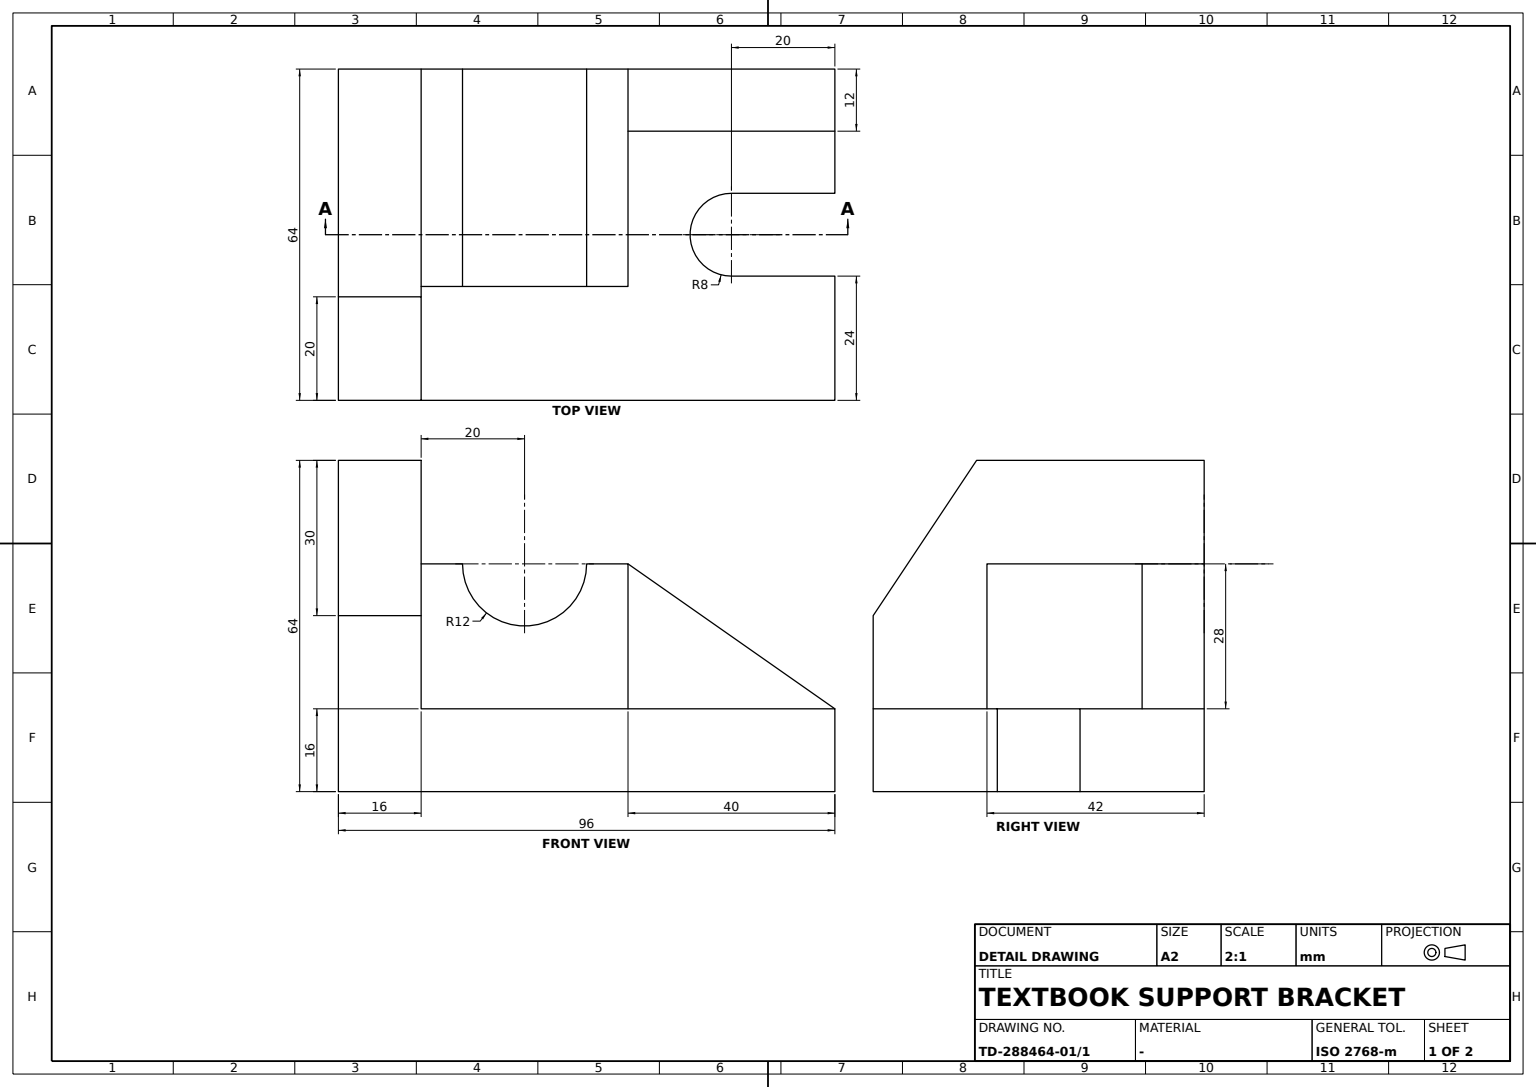
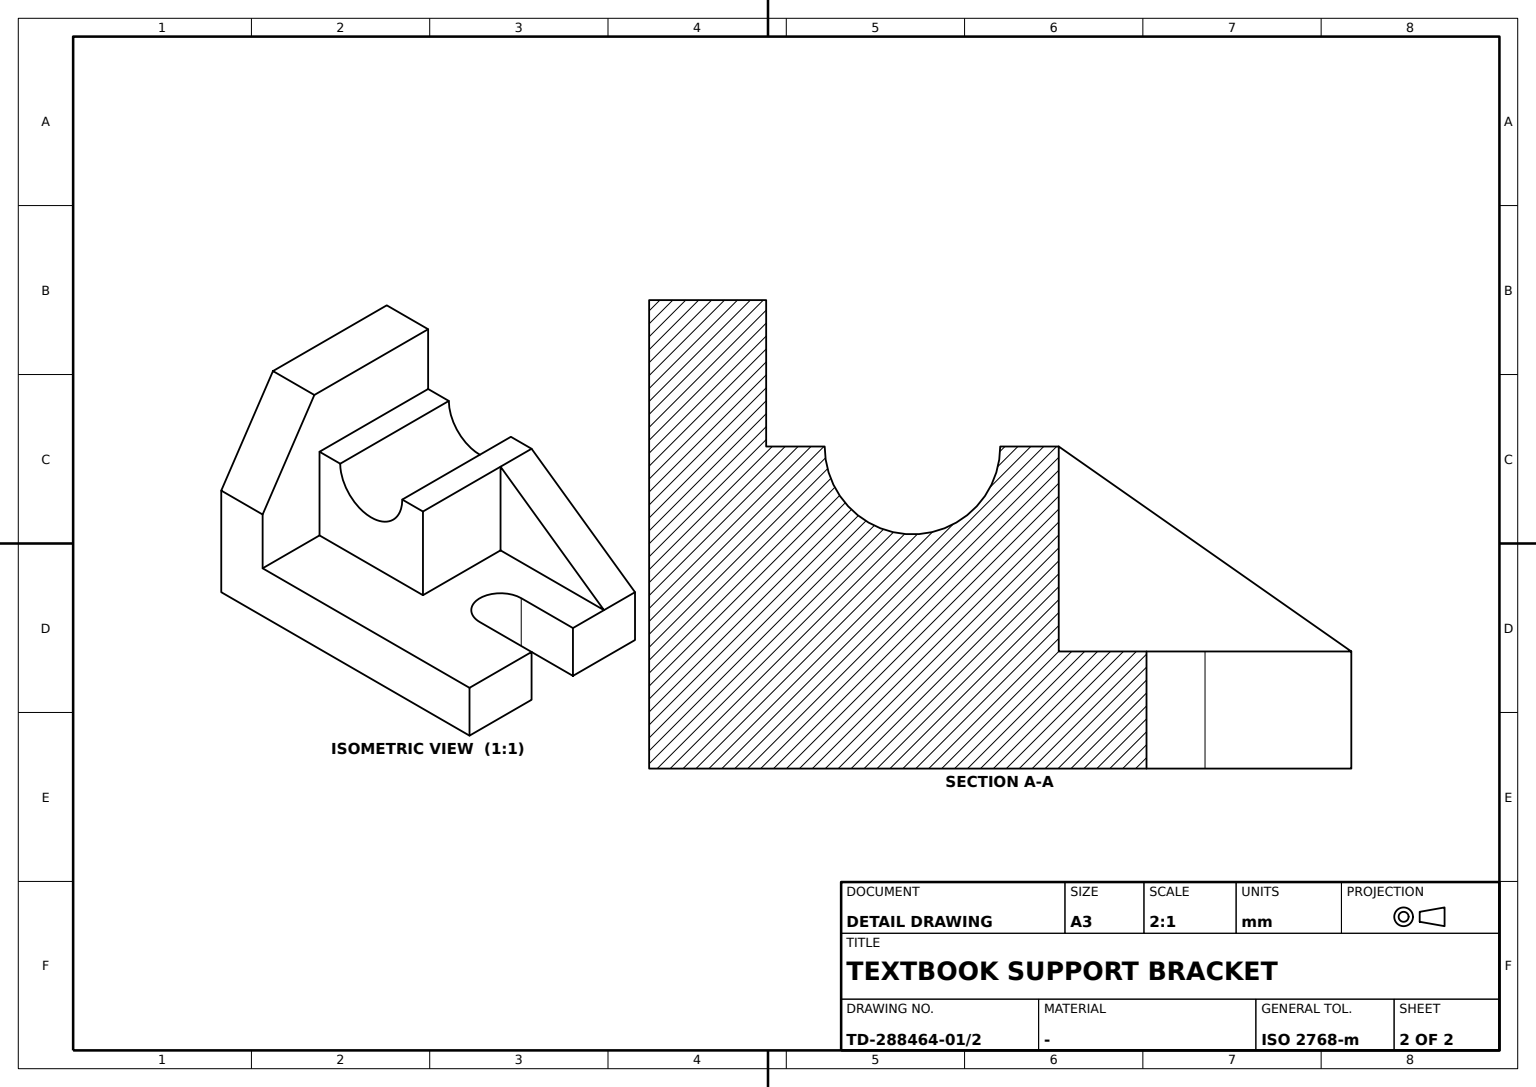
CATIA V5 part; units mm, degrees
sketch "Sketch1" plane through (0, 0, 0) normal (1, 0, 0) x (0, 1, 0)
  point P0 (-32.1888, 8.3831)
  point P1 (-48, -8)
  line L0 (-48, -8) -> (48, -8)
  line L1 (48, -8) -> (48, 8)
  line L2 (48, 8) -> (-48, 8)
  point P2 (-48, 8)
  line L3 (-48, 8) -> (-48, -8)
  point P3 (-48, 8)
  point P4 (-48, -8)
  dimension "length L1" = 16
  dimension "length L0" = 96
  constraint horizontal L0 x-axis
  constraint horizontal L2 x-axis
  constraint vertical L1 y-axis
  constraint vertical L3 y-axis
  constraint symmetry L2 L0 x-axis
  constraint symmetry L3 L1 y-axis
  constraint coincidence P3 L2
  constraint coincidence P4 L0
  constraint coincidence P3 P2
  constraint coincidence P1 P4
extrude "Pad1" add sketch "Sketch1" along normal mid plane 64
sketch "Sketch2" plane through (0, 0, 8) normal (0, 0, 1) x (1, 0, 0)
  arc A0 (-8, 28) -> (8, 28) centre (0, 28) ccw
  point P0 (0, 28)
  point P1 (8, 28)
  line L0 (8, 28) -> (8, 48)
  line L1 (8, 48) -> (-8, 48)
  line L2 (-8, 48) -> (-8, 28)
  point P2 (-8, 28)
  line L3 (-32, 48) -> (32, 48) construction
  line L4 (-32, 48) -> (32, 48) construction
  point P3 (-8, 28)
  point P4 (8, 28)
  dimension "radius A0" = 8
  dimension "distance P0 L4" = 20
  dimension "length L1" = 16
  constraint coincidence P0 y-axis
  constraint coincidence P1 A0
  constraint coincidence P2 A0
  constraint coincidence L1 L3
  constraint coincidence L0 P4
  constraint coincidence L2 P3
  constraint coincidence P1 P4
  constraint coincidence P2 P3
  constraint vertical L0 y-axis
  constraint vertical L2 y-axis
  constraint horizontal L1 x-axis
extrude "Pocket1" cut sketch "Sketch2" against normal blind 32
sketch "Sketch3" plane through (0, -48, 0) normal (0, -1, 0) x (1, 0, 0)
  line L0 (-32, 8) -> (-32, 56)
  line L1 (-32, 56) -> (12, 56)
  point P0 (12, 56)
  line L2 (12, 56) -> (32, 26)
  point P1 (32, 26)
  line L3 (32, 26) -> (32, 8)
  point P2 (32, 8)
  line L4 (32, 8) -> (-32, 8)
  line L5 (-32, 8) -> (32, 8) construction
  line L6 (32, 8) -> (32, -8) construction
  dimension "length L4" = 64
  dimension "distance P0 P1 y axis" = 30
  dimension "distance P1 P0 x axis" = 20
  dimension "length L0" = 48
  constraint vertical L0 y-axis
  constraint vertical L3 y-axis
  constraint horizontal L1 x-axis
  constraint horizontal L4 x-axis
  constraint coincidence L4 L5
  constraint coincidence P2 L6
extrude "Pad2" add sketch "Sketch3" against normal blind 16
sketch "Sketch4" plane through (-32, 0, 0) normal (-1, 0, 0) x (0, -1, 0)
  line L0 (-8, 36) -> (-8, 8)
  line L1 (-8, 8) -> (32, 8)
  line L2 (32, 8) -> (32, 36)
  line L3 (32, 36) -> (24, 36)
  point P0 (24, 36)
  line L4 (-8, 36) -> (0, 36)
  point P1 (0, 36)
  arc A0 (0, 36) -> (24, 36) centre (12, 36) ccw
  point P2 (12, 36)
  line L5 (32, 56) -> (32, 8) construction
  line L6 (-48, 8) -> (48, 8) construction
  point P3 (0, 36)
  point P4 (24, 36)
  dimension "radius A0" = 12
  dimension "distance L2 L0" = 40
  dimension "length L4" = 8
  dimension "length L3" = 8
  dimension "length L0" = 28
  constraint vertical L0 y-axis
  constraint vertical L2 y-axis
  constraint horizontal L1 x-axis
  constraint horizontal L3 x-axis
  constraint horizontal L4 x-axis
  constraint coincidence P2 L3
  constraint coincidence L2 L5
  constraint coincidence P1 A0
  constraint coincidence P0 A0
  constraint coincidence L1 L6
  constraint coincidence L3 P4
  constraint coincidence L4 P3
  constraint coincidence P0 P4
  constraint coincidence P1 P3
extrude "Pad3" add sketch "Sketch4" against normal blind 42
sketch "Sketch5" plane through (-32, 0, 0) normal (-1, 0, 0) x (0, -1, 0)
  line L0 (-48, 8) -> (-8, 36)
  point P0 (-48, 8)
  point P1 (-8, 36)
  line L1 (-48, 8) -> (-8, 8)
  point P2 (-48, 8)
  line L2 (-8, 36) -> (-8, 8)
  point P3 (-8, 36)
  constraint coincidence P2 P0
  constraint coincidence P3 P1
extrude "Pad4" add sketch "Sketch5" against normal blind 12
